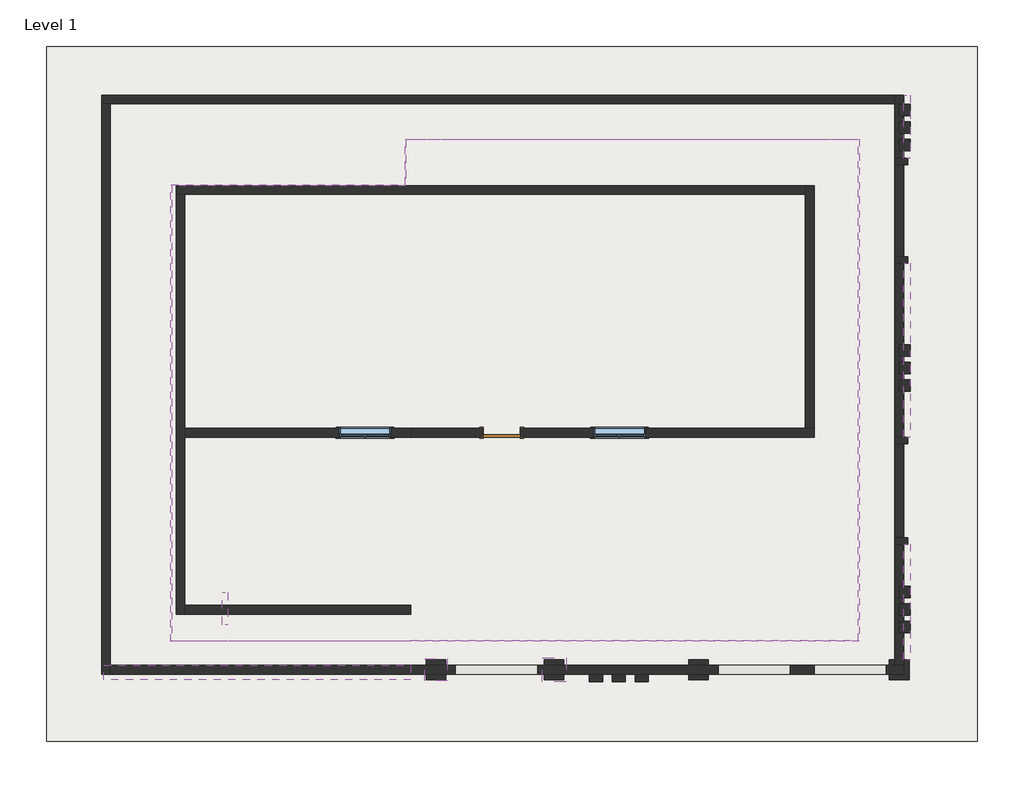
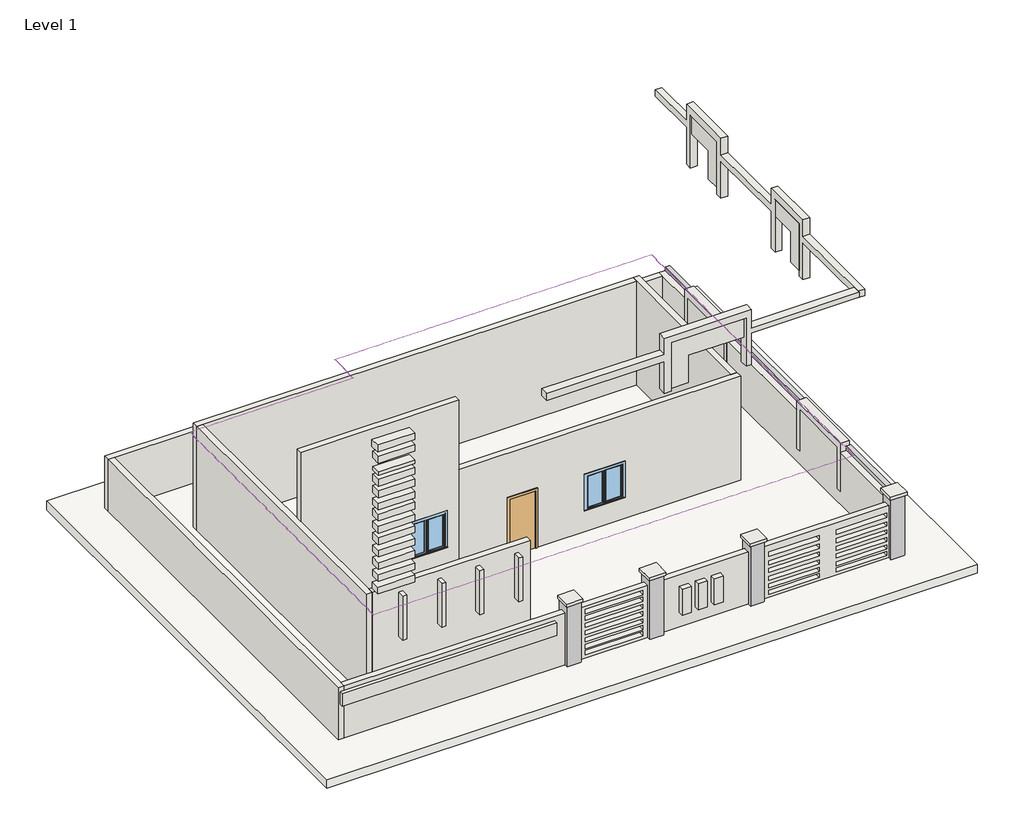
# One storey: 16 walls, 4 columns, 3 proxies, 2 coverings, 2 windows, 1 door, 1 slab.
"""IFC4 building model written with IfcOpenShell, lengths in millimetres."""

from ifc_helpers import new_model, si_unit, frame, origin, origin_with_axes, place, context, project, spatial, polyline, outline, extrude, faceted_brep, transform, mapped, element, save
from components import door_10fd3a06, walls_10_walls_10_12dc5ecd, walls_11_walls_11_b291a2b5, walls_12_walls_12_bacc6a5f, walls_13_walls_13_75e322be, walls_14_walls_14_a3be32cb, walls_2_walls_2_7a041f15, window_0862ab64

model = new_model("IFC4")

# Units and contexts
model_context = context("Model", 3, world=origin())
ifc_project = project(units=[si_unit("LENGTHUNIT", "METRE", prefix="MILLI")], contexts=[model_context])

# Site, building, storey
site = spatial("IfcSite", under=ifc_project)
building = spatial("IfcBuilding", under=site)
storey = spatial("IfcBuildingStorey", under=building, Name="Level 1", Elevation=0.0)

# Proxies
placement = place(None, origin())
element("IfcBuildingElementProxy", 1, Name="Cornice", ObjectType="Cornice", at=placement, inside=storey, context=model_context, shape_type="SweptSolid", body=[
    extrude(outline(polyline([(3201.2074298, -1465.8259649), (3353.6074298, -1465.8259649), (3353.6074298, -4158.7213241), (3201.2074298, -4158.7213241), (3201.2074298, -1465.8259649)])), frame((0.0, 0.0, 1828.8), z_axis=(0.0, 0.0, 1.0), x_axis=(1.0, 0.0, 0.0)), (0.0, 0.0, 1.0), 152.4),
])
element("IfcBuildingElementProxy", 2, Name="Cornice", ObjectType="Cornice", at=placement, inside=storey, context=model_context, shape_type="SweptSolid", body=[
    extrude(outline(polyline([(3201.2074298, 5061.9740351), (3353.6074298, 5061.9740351), (3353.6074298, 1023.3740351), (3201.2074298, 1023.3740351), (3201.2074298, 5061.9740351)])), frame((0.0, 0.0, 1828.8), z_axis=(0.0, 0.0, 1.0), x_axis=(1.0, 0.0, 0.0)), (0.0, 0.0, 1.0), 152.4),
])
element("IfcBuildingElementProxy", 3, Name="Cornice", ObjectType="Cornice", at=placement, inside=storey, context=model_context, shape_type="SweptSolid", body=[
    extrude(outline(polyline([(3201.2074298, 8973.0786759), (3353.6074298, 8973.0786759), (3353.6074298, 7499.8786759), (3201.2074298, 7499.8786759), (3201.2074298, 8973.0786759)])), frame((0.0, 0.0, 1785.441431), z_axis=(0.0, 0.0, 1.0), x_axis=(1.0, 0.0, 0.0)), (0.0, 0.0, 1.0), 152.4),
])

# Columns
element("IfcColumn", 4, ObjectType="Rectangular Column : 18\" x 18\"", at=placement, inside=storey, context=model_context, shape_type="SweptSolid", body=[
    extrude(outline(polyline([(-4615.9213241, 2133.6), (-4158.7213241, 2133.6), (-4158.7213241, 0.0), (-4285.7213241, 0.0), (-4285.7213241, 1828.8), (-4488.9213241, 1828.8), (-4488.9213241, 0.0), (-4615.9213241, 0.0), (-4615.9213241, 2133.6)])), frame((-7895.1305193, 0.0, 0.0), z_axis=(1.0, 0.0, 0.0), x_axis=(0.0, 1.0, 0.0)), (0.0, 0.0, 1.0), 457.2),
])
element("IfcColumn", 5, ObjectType="Rectangular Column : 18\" x 18\"", at=placement, inside=storey, context=model_context, shape_type="SweptSolid", body=[
    extrude(outline(polyline([(-4615.9213241, 2133.6), (-4158.7213241, 2133.6), (-4158.7213241, 0.0), (-4285.7213241, 0.0), (-4285.7213241, 1828.8), (-4488.9213241, 1828.8), (-4488.9213241, 0.0), (-4615.9213241, 0.0), (-4615.9213241, 2133.6)])), frame((-5151.9305193, 0.0, 0.0), z_axis=(1.0, 0.0, 0.0), x_axis=(0.0, 1.0, 0.0)), (0.0, 0.0, 1.0), 457.2),
])
element("IfcColumn", 6, ObjectType="Rectangular Column : 18\" x 18\"", at=placement, inside=storey, context=model_context, shape_type="SweptSolid", body=[
    extrude(outline(polyline([(-4615.9213241, 2133.6), (-4158.7213241, 2133.6), (-4158.7213241, 0.0), (-4285.7213241, 0.0), (-4285.7213241, 1828.8), (-4488.9213241, 1828.8), (-4488.9213241, 0.0), (-4615.9213241, 0.0), (-4615.9213241, 2133.6)])), frame((-1799.1305193, 0.0, 0.0), z_axis=(1.0, 0.0, 0.0), x_axis=(0.0, 1.0, 0.0)), (0.0, 0.0, 1.0), 457.2),
])
element("IfcColumn", 7, ObjectType="Rectangular Column : 18\" x 18\"", at=placement, inside=storey, context=model_context, shape_type="Brep", body=[
    faceted_brep([(3328.2074298, -4158.7213241, 2133.6), (2871.0074298, -4158.7213241, 2133.6), (2871.0074298, -4615.9213241, 2133.6), (3328.2074298, -4615.9213241, 2133.6), (2871.0074298, -4285.7213241, 0.0), (2871.0074298, -4158.7213241, 0.0), (2998.0074298, -4158.7213241, 0.0), (2998.0074298, -4285.7213241, 0.0), (3328.2074298, -4158.7213241, 0.0), (3201.2074298, -4158.7213241, 0.0), (3201.2074298, -4158.7213241, 1828.8), (2998.0074298, -4158.7213241, 1828.8), (2871.0074298, -4285.7213241, 1828.8), (2871.0074298, -4488.9213241, 1828.8), (2871.0074298, -4488.9213241, 0.0), (2871.0074298, -4615.9213241, 0.0), (3328.2074298, -4615.9213241, 0.0), (2998.0074298, -4285.7213241, 1828.8), (3201.2074298, -4488.9213241, 1828.8), (3201.2074298, -4488.9213241, 0.0), (3201.2074298, -4285.7213241, 1828.8), (3201.2074298, -4285.7213241, 0.0)], [[[0, 1, 2, 3]], [[4, 5, 6, 7]], [[1, 0, 8, 9, 10, 11, 6, 5]], [[2, 1, 5, 4, 12, 13, 14, 15]], [[3, 2, 15, 16]], [[0, 3, 16, 8]], [[12, 4, 7, 17]], [[18, 19, 14, 13]], [[19, 18, 20, 21]], [[11, 17, 7, 6]], [[20, 10, 9, 21]], [[8, 16, 15, 14, 19, 21, 9]], [[18, 13, 12, 17, 20]], [[17, 11, 10, 20]]]),
])

# Coverings
element("IfcCovering", 8, ObjectType="Fascia-Flat 1x12", at=placement, inside=storey, context=model_context, shape_type="Brep", body=[
    faceted_brep([(-8249.5228698, -3720.0759649, 3657.6), (-8249.5228698, -3707.3759649, 3657.6), (-8249.5228698, -3701.0259649, 3657.6), (-8249.5228698, -3701.0259649, 3371.85), (-8249.5228698, -3707.3759649, 3371.85), (-8249.5228698, -3720.0759649, 3371.85), (2164.4771302, -3720.0759649, 3657.6), (2145.4271302, -3701.0259649, 3657.6), (2145.4271302, -3701.0259649, 3371.85), (2164.4771302, -3720.0759649, 3371.85), (2164.4771302, 7951.2240351, 3657.6), (2145.4271302, 7932.1740351, 3657.6), (2145.4271302, 7932.1740351, 3371.85), (2164.4771302, 7951.2240351, 3371.85), (-8389.2228698, 7951.2240351, 3657.6), (-8370.1728698, 7932.1740351, 3657.6), (-8370.1728698, 7932.1740351, 3371.85), (-8389.2228698, 7951.2240351, 3371.85), (-8389.2228698, 6884.4240351, 3657.6), (-8370.1728698, 6865.3740351, 3657.6), (-8370.1728698, 6865.3740351, 3371.85), (-8389.2228698, 6884.4240351, 3371.85), (-13832.3805193, 6884.4240351, 3657.6), (-13813.3305193, 6865.3740351, 3657.6), (-13813.3305193, 6865.3740351, 3371.85), (-13832.3805193, 6884.4240351, 3371.85), (-13832.3805193, -3726.4259649, 3657.6), (-13832.3805193, -3726.4259649, 3371.85), (-13813.3305193, -3707.3759649, 3371.85), (-13813.3305193, -3707.3759649, 3657.6)], [[[0, 1, 2, 3, 4, 5]], [[2, 1, 0, 6, 7]], [[3, 2, 7, 8]], [[5, 4, 3, 8, 9]], [[0, 5, 9, 6]], [[7, 6, 10, 11]], [[8, 7, 11, 12]], [[9, 8, 12, 13]], [[6, 9, 13, 10]], [[11, 10, 14, 15]], [[12, 11, 15, 16]], [[13, 12, 16, 17]], [[10, 13, 17, 14]], [[15, 14, 18, 19]], [[16, 15, 19, 20]], [[17, 16, 20, 21]], [[14, 17, 21, 18]], [[19, 18, 22, 23]], [[20, 19, 23, 24]], [[21, 20, 24, 25]], [[18, 21, 25, 22]], [[26, 27, 28, 29]], [[23, 22, 26, 29]], [[24, 23, 29, 28]], [[25, 24, 28, 27]], [[22, 25, 27, 26]]]),
])
element("IfcCovering", 9, ObjectType="Fascia-Flat 1x12", at=placement, inside=storey, context=model_context, shape_type="Brep", body=[
    faceted_brep([(-13832.3805193, -3726.4259649, 3657.6), (-13813.3305193, -3707.3759649, 3657.6), (-13813.3305193, -3707.3759649, 3371.85), (-13832.3805193, -3726.4259649, 3371.85), (-8249.5228698, -3726.4259649, 3657.6), (-8249.5228698, -3726.4259649, 3371.85), (-8249.5228698, -3720.0759649, 3371.85), (-8249.5228698, -3707.3759649, 3371.85), (-8249.5228698, -3707.3759649, 3657.6), (-8249.5228698, -3720.0759649, 3657.6)], [[[0, 1, 2, 3]], [[4, 5, 6, 7, 8, 9]], [[1, 0, 4, 9, 8]], [[2, 1, 8, 7]], [[3, 2, 7, 6, 5]], [[0, 3, 5, 4]]]),
])

# Door
door_shape = door_10fd3a06(model_context)
element("IfcDoor", 10, ObjectType="Door-Single-Panel : 34\" x 80\"", at=placement, inside=storey, context=model_context, shape_type="MappedRepresentation", body=[
    mapped(door_shape, transform((-6142.5305193, 1124.9740351, 0.0), x_axis=(-1.0, 0.0, 0.0), y_axis=(0.0, -1.0, 0.0), z_axis=(0.0, 0.0, 1.0))),
])

# Slab
element("IfcSlab", 11, ObjectType="Generic - 12\"", at=placement, inside=storey, context=model_context, shape_type="SweptSolid", body=[
    extrude(outline(polyline([(4918.0010577, 10101.1985991), (4918.0010577, -6053.2014009), (-16722.7989423, -6053.2014009), (-16722.7989423, 10101.1985991), (4918.0010577, 10101.1985991)])), frame((0.0, 0.0, -304.8), z_axis=(0.0, 0.0, 1.0), x_axis=(1.0, 0.0, 0.0)), (0.0, 0.0, 1.0), 304.8),
])

# Walls
element("IfcWall", 12, ObjectType="Generic - 8\"", at=placement, inside=storey, context=model_context, shape_type="Brep", body=[
    faceted_brep([(-13711.7305193, 6662.1740351, 0.0), (-13508.5305193, 6662.1740351, 0.0), (918.6694807, 6662.1740351, 0.0), (918.6694807, 6662.1740351, 3657.6), (-13508.5305193, 6662.1740351, 3657.6), (-13711.7305193, 6662.1740351, 3657.6), (-13711.7305193, 6865.3740351, 0.0), (-13711.7305193, 6865.3740351, 3657.6), (-8370.1728698, 6865.3740351, 3657.6), (918.6694807, 6865.3740351, 3657.6), (918.6694807, 6865.3740351, 0.0)], [[[0, 1, 2, 3, 4, 5]], [[6, 7, 8, 9, 10]], [[2, 1, 0, 6, 10]], [[0, 5, 7, 6]], [[3, 2, 10, 9]], [[5, 4, 3, 9, 8, 7]]]),
])
element("IfcWall", 13, ObjectType="Generic - 8\"", at=placement, inside=storey, context=model_context, shape_type="Brep", body=[
    faceted_brep([(-13508.5305193, -3091.4259649, 0.0), (-13508.5305193, -2888.2259649, 0.0), (-13508.5305193, 1023.3740351, 0.0), (-13508.5305193, 1226.5740351, 0.0), (-13508.5305193, 6662.1740351, 0.0), (-13508.5305193, 6662.1740351, 3657.6), (-13508.5305193, -2888.2259649, 3657.6), (-13508.5305193, -3091.4259649, 3657.6), (-13711.7305193, -3091.4259649, 0.0), (-13711.7305193, -3091.4259649, 3657.6), (-13711.7305193, 6662.1740351, 3657.6), (-13711.7305193, 6662.1740351, 0.0)], [[[0, 1, 2, 3, 4, 5, 6, 7]], [[8, 9, 10, 11]], [[4, 3, 2, 1, 0, 8, 11]], [[0, 7, 9, 8]], [[5, 4, 11, 10]], [[7, 6, 5, 10, 9]]]),
])
element("IfcWall", 14, ObjectType="Generic - 8\"", at=placement, inside=storey, context=model_context, shape_type="SweptSolid", body=[
    extrude(outline(polyline([(-13508.5305193, -2888.2259649), (-8250.7305193, -2888.2259649), (-8250.7305193, -3091.4259649), (-13508.5305193, -3091.4259649), (-13508.5305193, -2888.2259649)])), origin_with_axes(), (0.0, 0.0, 1.0), 3657.6),
])
element("IfcWall", 15, ObjectType="Generic - 8\"", at=placement, inside=storey, context=model_context, shape_type="Brep", body=[
    faceted_brep([(918.6694807, 6865.3740351, 0.0), (918.6694807, 6662.1740351, 0.0), (918.6694807, 1226.5740351, 0.0), (918.6694807, 1226.5740351, 3657.6), (918.6694807, 6662.1740351, 3657.6), (918.6694807, 6865.3740351, 3657.6), (1121.8694807, 6865.3740351, 0.0), (1121.8694807, 6865.3740351, 3657.6), (1121.8694807, 1226.5740351, 3657.6), (1121.8694807, 1226.5740351, 0.0)], [[[0, 1, 2, 3, 4, 5]], [[6, 7, 8, 9]], [[2, 1, 0, 6, 9]], [[0, 5, 7, 6]], [[5, 4, 3, 8, 7]], [[3, 2, 9, 8]]]),
])
element("IfcWall", 16, ObjectType="Generic - 8\"", at=placement, inside=storey, context=model_context, shape_type="Brep", body=[
    faceted_brep([(-8250.7305193, 1023.3740351, 0.0), (-6574.3305193, 1023.3740351, 0.0), (-6574.3305193, 1023.3740351, 2032.0), (-5710.7305193, 1023.3740351, 2032.0), (-5710.7305193, 1023.3740351, 0.0), (1121.8694807, 1023.3740351, 0.0), (1121.8694807, 1023.3740351, 3657.6), (-8250.7305193, 1023.3740351, 3657.6), (-4008.9305193, 1023.3740351, 1960.9254934), (-2789.7305193, 1023.3740351, 1960.9254934), (-2789.7305193, 1023.3740351, 741.7254934), (-4008.9305193, 1023.3740351, 741.7254934), (-6574.3305193, 1226.5740351, 2032.0), (-6574.3305193, 1226.5740351, 0.0), (-8250.7305193, 1226.5740351, 0.0), (-8250.7305193, 1226.5740351, 3657.6), (918.6694807, 1226.5740351, 3657.6), (1121.8694807, 1226.5740351, 3657.6), (1121.8694807, 1226.5740351, 0.0), (918.6694807, 1226.5740351, 0.0), (-5710.7305193, 1226.5740351, 0.0), (-5710.7305193, 1226.5740351, 2032.0), (-4008.9305193, 1226.5740351, 1960.9254934), (-4008.9305193, 1226.5740351, 741.7254934), (-2789.7305193, 1226.5740351, 741.7254934), (-2789.7305193, 1226.5740351, 1960.9254934)], [[[0, 1, 2, 3, 4, 5, 6, 7], [8, 9, 10, 11]], [[12, 13, 14, 15, 16, 17, 18, 19, 20, 21], [22, 23, 24, 25]], [[14, 13, 1, 0]], [[20, 19, 18, 5, 4]], [[7, 6, 17, 16, 15]], [[0, 7, 15, 14]], [[6, 5, 18, 17]], [[23, 22, 8, 11]], [[24, 23, 11, 10]], [[25, 24, 10, 9]], [[22, 25, 9, 8]], [[2, 1, 13, 12]], [[3, 2, 12, 21]], [[4, 3, 21, 20]]]),
])
element("IfcWall", 17, ObjectType="Generic - 8\"", at=placement, inside=storey, context=model_context, shape_type="Brep", body=[
    faceted_brep([(-8250.7305193, 1226.5740351, 0.0), (-13508.5305193, 1226.5740351, 0.0), (-13508.5305193, 1226.5740351, 6096.0), (-8250.7305193, 1226.5740351, 6096.0), (-8250.7305193, 1226.5740351, 3657.6), (-9927.1305193, 1226.5740351, 2285.1492606), (-9927.1305193, 1226.5740351, 1065.9492606), (-8707.9305193, 1226.5740351, 1065.9492606), (-8707.9305193, 1226.5740351, 2285.1492606), (-8250.7305193, 1023.3740351, 0.0), (-8250.7305193, 1023.3740351, 3657.6), (-8250.7305193, 1023.3740351, 6096.0), (-13508.5305193, 1023.3740351, 6096.0), (-13508.5305193, 1023.3740351, 0.0), (-9927.1305193, 1023.3740351, 2285.1492606), (-8707.9305193, 1023.3740351, 2285.1492606), (-8707.9305193, 1023.3740351, 1065.9492606), (-9927.1305193, 1023.3740351, 1065.9492606)], [[[0, 1, 2, 3, 4], [5, 6, 7, 8]], [[9, 10, 11, 12, 13], [14, 15, 16, 17]], [[1, 0, 9, 13]], [[3, 2, 12, 11]], [[0, 4, 3, 11, 10, 9]], [[2, 1, 13, 12]], [[6, 5, 14, 17]], [[7, 6, 17, 16]], [[8, 7, 16, 15]], [[5, 8, 15, 14]]]),
])
element("IfcWall", 18, ObjectType="Generic - 8\"", at=placement, inside=storey, context=model_context, shape_type="Brep", body=[
    faceted_brep([(-15442.3925702, 8769.8786759, 0.0), (-15239.1925702, 8769.8786759, 0.0), (2998.0074298, 8769.8786759, 0.0), (2998.0074298, 8769.8786759, 1828.8), (-15239.1925702, 8769.8786759, 1828.8), (-15442.3925702, 8769.8786759, 1828.8), (-15442.3925702, 8973.0786759, 0.0), (-15442.3925702, 8973.0786759, 1828.8), (2998.0074298, 8973.0786759, 1828.8), (2998.0074298, 8973.0786759, 0.0)], [[[0, 1, 2, 3, 4, 5]], [[6, 7, 8, 9]], [[2, 1, 0, 6, 9]], [[5, 4, 3, 8, 7]], [[0, 5, 7, 6]], [[3, 2, 9, 8]]]),
])
element("IfcWall", 19, ObjectType="Generic - 8\"", at=placement, inside=storey, context=model_context, shape_type="Brep", body=[
    faceted_brep([(-15239.1925702, -4488.9213241, 0.0), (-15239.1925702, -4285.7213241, 0.0), (-15239.1925702, 8769.8786759, 0.0), (-15239.1925702, 8769.8786759, 1828.8), (-15239.1925702, -4285.7213241, 1828.8), (-15239.1925702, -4488.9213241, 1828.8), (-15442.3925702, -4488.9213241, 0.0), (-15442.3925702, -4488.9213241, 1828.8), (-15442.3925702, 8769.8786759, 1828.8), (-15442.3925702, 8769.8786759, 0.0)], [[[0, 1, 2, 3, 4, 5]], [[6, 7, 8, 9]], [[2, 1, 0, 6, 9]], [[5, 4, 3, 8, 7]], [[0, 5, 7, 6]], [[3, 2, 9, 8]]]),
])
element("IfcWall", 20, ObjectType="Generic - 8\"", at=placement, inside=storey, context=model_context, shape_type="Brep", body=[
    faceted_brep([(3201.2074298, -4285.7213241, 0.0), (2998.0074298, -4285.7213241, 0.0), (2871.0074298, -4285.7213241, 0.0), (-1341.9305193, -4285.7213241, 0.0), (-1799.1305193, -4285.7213241, 0.0), (-4694.7305193, -4285.7213241, 0.0), (-5151.9305193, -4285.7213241, 0.0), (-7437.9305193, -4285.7213241, 0.0), (-7895.1305193, -4285.7213241, 0.0), (-15239.1925702, -4285.7213241, 0.0), (-15239.1925702, -4285.7213241, 1828.8), (-7895.1305193, -4285.7213241, 1828.8), (-7437.9305193, -4285.7213241, 1828.8), (-5151.9305193, -4285.7213241, 1828.8), (-4694.7305193, -4285.7213241, 1828.8), (-1799.1305193, -4285.7213241, 1828.8), (-1341.9305193, -4285.7213241, 1828.8), (2871.0074298, -4285.7213241, 1828.8), (2998.0074298, -4285.7213241, 1828.8), (3201.2074298, -4285.7213241, 1828.8), (2798.2694807, -4285.7213241, 1590.6295089), (1121.8694807, -4285.7213241, 1590.6295089), (1121.8694807, -4285.7213241, 1438.2295089), (2798.2694807, -4285.7213241, 1438.2295089), (2798.2694807, -4285.7213241, 1285.530341), (1121.8694807, -4285.7213241, 1285.530341), (1121.8694807, -4285.7213241, 1133.7858691), (2798.2694807, -4285.7213241, 1133.7858691), (2798.2694807, -4285.7213241, 1009.753772), (1121.8694807, -4285.7213241, 1009.753772), (1121.8694807, -4285.7213241, 869.7393415), (2798.2694807, -4285.7213241, 869.7393415), (2798.2694807, -4285.7213241, 736.2637339), (1121.8694807, -4285.7213241, 736.2637339), (1121.8694807, -4285.7213241, 596.2533887), (2798.2694807, -4285.7213241, 596.2533887), (2798.2694807, -4285.7213241, 467.4688962), (1121.8694807, -4285.7213241, 467.4688962), (1121.8694807, -4285.7213241, 327.4258682), (2798.2694807, -4285.7213241, 327.4258682), (2798.2694807, -4285.7213241, 250.5459581), (1121.8694807, -4285.7213241, 250.5459581), (1121.8694807, -4285.7213241, 105.8322418), (2798.2694807, -4285.7213241, 105.8322418), (563.0694807, -4285.7213241, 1590.6295089), (-1113.3305193, -4285.7213241, 1590.6295089), (-1113.3305193, -4285.7213241, 1438.2295089), (563.0694807, -4285.7213241, 1438.2295089), (563.0694807, -4285.7213241, 1285.530341), (-1113.3305193, -4285.7213241, 1285.530341), (-1113.3305193, -4285.7213241, 1133.7858691), (563.0694807, -4285.7213241, 1133.7858691), (563.0694807, -4285.7213241, 1009.753772), (-1113.3305193, -4285.7213241, 1009.753772), (-1113.3305193, -4285.7213241, 869.7393415), (563.0694807, -4285.7213241, 869.7393415), (563.0694807, -4285.7213241, 736.2637339), (-1113.3305193, -4285.7213241, 736.2637339), (-1113.3305193, -4285.7213241, 596.2533887), (563.0694807, -4285.7213241, 596.2533887), (563.0694807, -4285.7213241, 467.4688962), (-1113.3305193, -4285.7213241, 467.4688962), (-1113.3305193, -4285.7213241, 327.4258682), (563.0694807, -4285.7213241, 327.4258682), (563.0694807, -4285.7213241, 250.5459581), (-1113.3305193, -4285.7213241, 250.5459581), (-1113.3305193, -4285.7213241, 105.8322418), (563.0694807, -4285.7213241, 105.8322418), (-5305.1552948, -4285.7213241, 1704.9295089), (-7219.390028, -4285.7213241, 1704.9295089), (-7219.390028, -4285.7213241, 1552.5295089), (-5305.1552948, -4285.7213241, 1552.5295089), (-5305.1552948, -4285.7213241, 1225.653772), (-7219.390028, -4285.7213241, 1225.653772), (-7219.390028, -4285.7213241, 1073.253772), (-5305.1552948, -4285.7213241, 1073.253772), (-5305.1552948, -4285.7213241, 964.8637339), (-7219.390028, -4285.7213241, 964.8637339), (-7219.390028, -4285.7213241, 812.4637339), (-5305.1552948, -4285.7213241, 812.4637339), (-5305.1552948, -4285.7213241, 715.1188962), (-7219.390028, -4285.7213241, 715.1188962), (-7219.390028, -4285.7213241, 562.7188962), (-5305.1552948, -4285.7213241, 562.7188962), (-5305.1552948, -4285.7213241, 479.1459581), (-7219.390028, -4285.7213241, 479.1459581), (-7219.390028, -4285.7213241, 326.7459581), (-5305.1552948, -4285.7213241, 326.7459581), (-5305.1552948, -4285.7213241, 1476.3295089), (-7219.390028, -4285.7213241, 1476.3295089), (-7219.390028, -4285.7213241, 1323.9295089), (-5305.1552948, -4285.7213241, 1323.9295089), (-5305.1552948, -4285.7213241, 263.2459581), (-7219.390028, -4285.7213241, 263.2459581), (-7219.390028, -4285.7213241, 110.8459581), (-5305.1552948, -4285.7213241, 110.8459581), (3201.2074298, -4488.9213241, 0.0), (3201.2074298, -4488.9213241, 1828.8), (2871.0074298, -4488.9213241, 1828.8), (-1341.9305193, -4488.9213241, 1828.8), (-1799.1305193, -4488.9213241, 1828.8), (-4694.7305193, -4488.9213241, 1828.8), (-5151.9305193, -4488.9213241, 1828.8), (-7437.9305193, -4488.9213241, 1828.8), (-7895.1305193, -4488.9213241, 1828.8), (-15239.1925702, -4488.9213241, 1828.8), (-15239.1925702, -4488.9213241, 0.0), (-7895.1305193, -4488.9213241, 0.0), (-7437.9305193, -4488.9213241, 0.0), (-5151.9305193, -4488.9213241, 0.0), (-4694.7305193, -4488.9213241, 0.0), (-1799.1305193, -4488.9213241, 0.0), (-1341.9305193, -4488.9213241, 0.0), (2871.0074298, -4488.9213241, 0.0), (2798.2694807, -4488.9213241, 1590.6295089), (2798.2694807, -4488.9213241, 1438.2295089), (1121.8694807, -4488.9213241, 1438.2295089), (1121.8694807, -4488.9213241, 1590.6295089), (2798.2694807, -4488.9213241, 1285.530341), (2798.2694807, -4488.9213241, 1133.7858691), (1121.8694807, -4488.9213241, 1133.7858691), (1121.8694807, -4488.9213241, 1285.530341), (2798.2694807, -4488.9213241, 1009.753772), (2798.2694807, -4488.9213241, 869.7393415), (1121.8694807, -4488.9213241, 869.7393415), (1121.8694807, -4488.9213241, 1009.753772), (2798.2694807, -4488.9213241, 736.2637339), (2798.2694807, -4488.9213241, 596.2533887), (1121.8694807, -4488.9213241, 596.2533887), (1121.8694807, -4488.9213241, 736.2637339), (2798.2694807, -4488.9213241, 467.4688962), (2798.2694807, -4488.9213241, 327.4258682), (1121.8694807, -4488.9213241, 327.4258682), (1121.8694807, -4488.9213241, 467.4688962), (2798.2694807, -4488.9213241, 250.5459581), (2798.2694807, -4488.9213241, 105.8322418), (1121.8694807, -4488.9213241, 105.8322418), (1121.8694807, -4488.9213241, 250.5459581), (563.0694807, -4488.9213241, 1590.6295089), (563.0694807, -4488.9213241, 1438.2295089), (-1113.3305193, -4488.9213241, 1438.2295089), (-1113.3305193, -4488.9213241, 1590.6295089), (563.0694807, -4488.9213241, 1285.530341), (563.0694807, -4488.9213241, 1133.7858691), (-1113.3305193, -4488.9213241, 1133.7858691), (-1113.3305193, -4488.9213241, 1285.530341), (563.0694807, -4488.9213241, 1009.753772), (563.0694807, -4488.9213241, 869.7393415), (-1113.3305193, -4488.9213241, 869.7393415), (-1113.3305193, -4488.9213241, 1009.753772), (563.0694807, -4488.9213241, 736.2637339), (563.0694807, -4488.9213241, 596.2533887), (-1113.3305193, -4488.9213241, 596.2533887), (-1113.3305193, -4488.9213241, 736.2637339), (563.0694807, -4488.9213241, 467.4688962), (563.0694807, -4488.9213241, 327.4258682), (-1113.3305193, -4488.9213241, 327.4258682), (-1113.3305193, -4488.9213241, 467.4688962), (563.0694807, -4488.9213241, 250.5459581), (563.0694807, -4488.9213241, 105.8322418), (-1113.3305193, -4488.9213241, 105.8322418), (-1113.3305193, -4488.9213241, 250.5459581), (-5305.1552948, -4488.9213241, 1704.9295089), (-5305.1552948, -4488.9213241, 1552.5295089), (-7219.390028, -4488.9213241, 1552.5295089), (-7219.390028, -4488.9213241, 1704.9295089), (-5305.1552948, -4488.9213241, 1225.653772), (-5305.1552948, -4488.9213241, 1073.253772), (-7219.390028, -4488.9213241, 1073.253772), (-7219.390028, -4488.9213241, 1225.653772), (-5305.1552948, -4488.9213241, 964.8637339), (-5305.1552948, -4488.9213241, 812.4637339), (-7219.390028, -4488.9213241, 812.4637339), (-7219.390028, -4488.9213241, 964.8637339), (-5305.1552948, -4488.9213241, 715.1188962), (-5305.1552948, -4488.9213241, 562.7188962), (-7219.390028, -4488.9213241, 562.7188962), (-7219.390028, -4488.9213241, 715.1188962), (-5305.1552948, -4488.9213241, 479.1459581), (-5305.1552948, -4488.9213241, 326.7459581), (-7219.390028, -4488.9213241, 326.7459581), (-7219.390028, -4488.9213241, 479.1459581), (-5305.1552948, -4488.9213241, 1476.3295089), (-5305.1552948, -4488.9213241, 1323.9295089), (-7219.390028, -4488.9213241, 1323.9295089), (-7219.390028, -4488.9213241, 1476.3295089), (-5305.1552948, -4488.9213241, 263.2459581), (-5305.1552948, -4488.9213241, 110.8459581), (-7219.390028, -4488.9213241, 110.8459581), (-7219.390028, -4488.9213241, 263.2459581)], [[[0, 1, 2, 3, 4, 5, 6, 7, 8, 9, 10, 11, 12, 13, 14, 15, 16, 17, 18, 19], [20, 21, 22, 23], [24, 25, 26, 27], [28, 29, 30, 31], [32, 33, 34, 35], [36, 37, 38, 39], [40, 41, 42, 43], [44, 45, 46, 47], [48, 49, 50, 51], [52, 53, 54, 55], [56, 57, 58, 59], [60, 61, 62, 63], [64, 65, 66, 67], [68, 69, 70, 71], [72, 73, 74, 75], [76, 77, 78, 79], [80, 81, 82, 83], [84, 85, 86, 87], [88, 89, 90, 91], [92, 93, 94, 95]], [[96, 97, 98, 99, 100, 101, 102, 103, 104, 105, 106, 107, 108, 109, 110, 111, 112, 113], [114, 115, 116, 117], [118, 119, 120, 121], [122, 123, 124, 125], [126, 127, 128, 129], [130, 131, 132, 133], [134, 135, 136, 137], [138, 139, 140, 141], [142, 143, 144, 145], [146, 147, 148, 149], [150, 151, 152, 153], [154, 155, 156, 157], [158, 159, 160, 161], [162, 163, 164, 165], [166, 167, 168, 169], [170, 171, 172, 173], [174, 175, 176, 177], [178, 179, 180, 181], [182, 183, 184, 185], [186, 187, 188, 189]], [[0, 19, 97, 96]], [[10, 9, 106, 105]], [[9, 8, 7, 6, 5, 4, 3, 2, 1, 0, 96, 113, 112, 111, 110, 109, 108, 107, 106]], [[19, 18, 17, 16, 15, 14, 13, 12, 11, 10, 105, 104, 103, 102, 101, 100, 99, 98, 97]], [[21, 20, 114, 117]], [[22, 21, 117, 116]], [[23, 22, 116, 115]], [[20, 23, 115, 114]], [[25, 24, 118, 121]], [[26, 25, 121, 120]], [[27, 26, 120, 119]], [[24, 27, 119, 118]], [[29, 28, 122, 125]], [[30, 29, 125, 124]], [[31, 30, 124, 123]], [[28, 31, 123, 122]], [[33, 32, 126, 129]], [[34, 33, 129, 128]], [[35, 34, 128, 127]], [[32, 35, 127, 126]], [[37, 36, 130, 133]], [[38, 37, 133, 132]], [[39, 38, 132, 131]], [[36, 39, 131, 130]], [[41, 40, 134, 137]], [[42, 41, 137, 136]], [[43, 42, 136, 135]], [[40, 43, 135, 134]], [[45, 44, 138, 141]], [[46, 45, 141, 140]], [[47, 46, 140, 139]], [[44, 47, 139, 138]], [[49, 48, 142, 145]], [[50, 49, 145, 144]], [[51, 50, 144, 143]], [[48, 51, 143, 142]], [[53, 52, 146, 149]], [[54, 53, 149, 148]], [[55, 54, 148, 147]], [[52, 55, 147, 146]], [[57, 56, 150, 153]], [[58, 57, 153, 152]], [[59, 58, 152, 151]], [[56, 59, 151, 150]], [[61, 60, 154, 157]], [[62, 61, 157, 156]], [[63, 62, 156, 155]], [[60, 63, 155, 154]], [[65, 64, 158, 161]], [[66, 65, 161, 160]], [[67, 66, 160, 159]], [[64, 67, 159, 158]], [[69, 68, 162, 165]], [[70, 69, 165, 164]], [[71, 70, 164, 163]], [[68, 71, 163, 162]], [[73, 72, 166, 169]], [[74, 73, 169, 168]], [[75, 74, 168, 167]], [[72, 75, 167, 166]], [[77, 76, 170, 173]], [[78, 77, 173, 172]], [[79, 78, 172, 171]], [[76, 79, 171, 170]], [[81, 80, 174, 177]], [[82, 81, 177, 176]], [[83, 82, 176, 175]], [[80, 83, 175, 174]], [[85, 84, 178, 181]], [[86, 85, 181, 180]], [[87, 86, 180, 179]], [[84, 87, 179, 178]], [[89, 88, 182, 185]], [[90, 89, 185, 184]], [[91, 90, 184, 183]], [[88, 91, 183, 182]], [[93, 92, 186, 189]], [[94, 93, 189, 188]], [[95, 94, 188, 187]], [[92, 95, 187, 186]]]),
])
element("IfcWall", 21, ObjectType="Generic - 8\"", at=placement, inside=storey, context=model_context, shape_type="Brep", body=[
    faceted_brep([(2998.0074298, 8973.0786759, 0.0), (2998.0074298, 8769.8786759, 0.0), (2998.0074298, -4158.7213241, 0.0), (2998.0074298, -4285.7213241, 0.0), (2998.0074298, -4285.7213241, 1828.8), (2998.0074298, -4158.7213241, 1828.8), (2998.0074298, -1465.8259649, 1828.8), (2998.0074298, -1465.8259649, 2133.6), (2998.0074298, 1023.3740351, 2133.6), (2998.0074298, 1023.3740351, 1828.8), (2998.0074298, 5061.4786759, 1828.8), (2998.0074298, 5061.4786759, 2133.6), (2998.0074298, 7499.8786759, 2133.6), (2998.0074298, 7499.8786759, 1828.8), (2998.0074298, 8769.8786759, 1828.8), (2998.0074298, 8973.0786759, 1828.8), (3201.2074298, 8973.0786759, 0.0), (3201.2074298, 8973.0786759, 1828.8), (3201.2074298, 7499.8786759, 1828.8), (3201.2074298, 7499.8786759, 2133.6), (3201.2074298, 5061.4786759, 2133.6), (3201.2074298, 5061.4786759, 1828.8), (3201.2074298, 1023.3740351, 1828.8), (3201.2074298, 1023.3740351, 2133.6), (3201.2074298, -1465.8259649, 2133.6), (3201.2074298, -1465.8259649, 1828.8), (3201.2074298, -4158.7213241, 1828.8), (3201.2074298, -4285.7213241, 1828.8), (3201.2074298, -4285.7213241, 0.0), (3201.2074298, -4158.7213241, 0.0)], [[[0, 1, 2, 3, 4, 5, 6, 7, 8, 9, 10, 11, 12, 13, 14, 15]], [[16, 17, 18, 19, 20, 21, 22, 23, 24, 25, 26, 27, 28, 29]], [[0, 15, 17, 16]], [[4, 3, 28, 27]], [[3, 2, 1, 0, 16, 29, 28]], [[6, 5, 4, 27, 26, 25]], [[7, 6, 25, 24]], [[8, 7, 24, 23]], [[9, 8, 23, 22]], [[10, 9, 22, 21]], [[11, 10, 21, 20]], [[12, 11, 20, 19]], [[13, 12, 19, 18]], [[15, 14, 13, 18, 17]]]),
])
walls_10_walls_10_shape = walls_10_walls_10_12dc5ecd(model_context)
element("IfcWall", 22, ObjectType="Walls 10 : Walls 10", at=placement, inside=storey, context=model_context, shape_type="MappedRepresentation", body=[
    mapped(walls_10_walls_10_shape, transform((0.0, 0.0, 0.0), x_axis=(1.0, 0.0, 0.0), y_axis=(0.0, 1.0, 0.0), z_axis=(0.0, 0.0, 1.0))),
])
walls_11_walls_11_shape = walls_11_walls_11_b291a2b5(model_context)
element("IfcWall", 23, ObjectType="Walls 11 : Walls 11", at=placement, inside=storey, context=model_context, shape_type="MappedRepresentation", body=[
    mapped(walls_11_walls_11_shape, transform((0.0, 0.0, 0.0), x_axis=(1.0, 0.0, 0.0), y_axis=(0.0, 1.0, 0.0), z_axis=(0.0, 0.0, 1.0))),
])
walls_12_walls_12_shape = walls_12_walls_12_bacc6a5f(model_context)
element("IfcWall", 24, ObjectType="Walls 12 : Walls 12", at=placement, inside=storey, context=model_context, shape_type="MappedRepresentation", body=[
    mapped(walls_12_walls_12_shape, transform((0.0, 0.0, 0.0), x_axis=(1.0, 0.0, 0.0), y_axis=(0.0, 1.0, 0.0), z_axis=(0.0, 0.0, 1.0))),
])
walls_13_walls_13_shape = walls_13_walls_13_75e322be(model_context)
element("IfcWall", 25, ObjectType="Walls 13 : Walls 13", at=placement, inside=storey, context=model_context, shape_type="MappedRepresentation", body=[
    mapped(walls_13_walls_13_shape, transform((0.0, 0.0, 0.0), x_axis=(1.0, 0.0, 0.0), y_axis=(0.0, 1.0, 0.0), z_axis=(0.0, 0.0, 1.0))),
])
walls_14_walls_14_shape = walls_14_walls_14_a3be32cb(model_context)
element("IfcWall", 26, ObjectType="Walls 14 : Walls 14", at=placement, inside=storey, context=model_context, shape_type="MappedRepresentation", body=[
    mapped(walls_14_walls_14_shape, transform((0.0, 0.0, 0.0), x_axis=(1.0, 0.0, 0.0), y_axis=(0.0, 1.0, 0.0), z_axis=(0.0, 0.0, 1.0))),
])
walls_2_walls_2_shape = walls_2_walls_2_7a041f15(model_context)
element("IfcWall", 27, ObjectType="Walls 2 : Walls 2", at=placement, inside=storey, context=model_context, shape_type="MappedRepresentation", body=[
    mapped(walls_2_walls_2_shape, transform((0.0, 0.0, 0.0), x_axis=(1.0, 0.0, 0.0), y_axis=(0.0, 1.0, 0.0), z_axis=(0.0, 0.0, 1.0))),
])

# Windows
window_shape = window_0862ab64(model_context)
element("IfcWindow", 28, ObjectType="Casement Dbl with Trim : 48\" x 48\"", at=placement, inside=storey, context=model_context, shape_type="MappedRepresentation", body=[
    mapped(window_shape, transform((-3399.3305193, 1144.0240351, -172.6745066), x_axis=(-1.0, 0.0, 0.0), y_axis=(0.0, -1.0, 0.0), z_axis=(0.0, 0.0, 1.0))),
])
element("IfcWindow", 29, ObjectType="Casement Dbl with Trim : 48\" x 48\"", at=placement, inside=storey, context=model_context, shape_type="MappedRepresentation", body=[
    mapped(window_shape, transform((-9317.5305193, 1144.0240351, 151.5492606), x_axis=(-1.0, 0.0, 0.0), y_axis=(0.0, -1.0, 0.0), z_axis=(0.0, 0.0, 1.0))),
])

save(model, "model.ifc")

# Revit data of these elements
# Type "Rectangular Column : 18\" x 18\""
#   Assembly Code = "B1010200"
#   Depth = 1' - 6"
#   Offset Base = 0' - 0"
#   Offset Top = 0' - 0"
#   Width = 1' - 6"
#   Material = none
# Type "Door-Single-Panel : 34\" x 80\""
#   Type Mark = "8"
#   Construction Type Id = "DOOR"
#   Assembly Code = "C1020300"
#   Analytic Construction = "Wooden"
#   Thickness = 0' - 2"
#   Thermal Resistance (R) = 2.5876 (h·ft²·°F)/BTU
#   Swing Angle [instance default] = 90.00°
#   Heat Transfer Coefficient (U) = 0.3865 BTU/(h·ft²·°F)
#   Height = 6' - 8"
#   Trim Projection Ext = 0' - 1"
#   Trim Projection Int = 0' - 1"
#   Trim Width = 0' - 3"
#   Width = 2' - 10"
#   Define Thermal Properties by = 1
#   Panel Material = Wood - Birch - Solid Stained Light Low Gloss
#   Trim Material = Roofing, EPDM Membrane
#   Visual Light Transmittance = 0
#   Solar Heat Gain Coefficient = 0
#   Function = (empty or 0)
#   Wall Closure = (empty or 0)
# Type "Generic - 12\""
#   Assembly Code = "B1010"
#   Function = 0
#   Layers, outside or top first: 1' - 0" no material (function 1)
# Type "Generic - 8\""
#   Assembly Code = "B2010"
#   Layers, outside or top first: 0' - 8" no material (function 1)
# Type "Casement Dbl with Trim : 48\" x 48\""
#   Type Mark = "19"
#   Construction Type Id = "GSP4R"
#   Assembly Code = "B2020100"
#   Analytic Construction = "1/8 in Pilkington single glazing"
#   Visual Light Transmittance = 0.9
#   Solar Heat Gain Coefficient = 0.78
#   Heat Transfer Coefficient (U) = 0.6496 BTU/(h·ft²·°F)
#   Height = 4' - 0"
#   Default Sill Height = 3' - 0"
#   Trim Projection - Ext. = 0' - 0 1/2"
#   Trim Projection - Int. = 0' - 0 3/4"
#   Trim Width - Exterior = 0' - 3 1/2"
#   Trim Width - Interior = 0' - 3 1/2"
#   Width = 4' - 0"
#   Window Inset = 0' - 0 3/4"
#   Define Thermal Properties by = 1
#   Glass Pane Material = Glass
#   Sash Material = Sash
#   Trim Exterior Material = Trim
#   Trim Interior Material = Trim
#   Wall Closure = (empty or 0)
# Elements 1, 2, 3 (IfcBuildingElementProxy, "Cornice")
#   Phase Created = New Construction
#   Materials on its faces: "Default Wall"
# Elements 4, 5, 6, 7 (IfcColumn, "Rectangular Column : 18\" x 18\"")
#   Phase Created = New Construction
#   Materials on its faces: "Default Wall"
# Elements 8, 9 (IfcCovering, "Fascia-Flat 1x12")
#   Phase Created = New Construction
#   Materials on its faces: "Default Roof"
# Element 10 (IfcDoor, "Door-Single-Panel : 34\" x 80\"")
#   Swing Angle = 90.00°
#   Phase Created = New Construction
#   Materials on its faces: "Roofing, EPDM Membrane", "Wood - Birch - Solid Stained Light Low Gloss"
# Element 11 (IfcSlab, "Generic - 12\"")
#   Height Offset From Level = 0' - 0"
#   Phase Created = New Construction
#   Materials on its faces: "Default Floor"
# Elements 12, 13, 14, 15, 16 (IfcWall, "Generic - 8\"")
#   Top Offset = 0' - 0"
#   Base Offset = 0' - 0"
#   Unconnected Height = 12' - 0"
#   wall height = 12' - 0"
#   Phase Created = New Construction
#   Base Constraint = Level 1
#   Materials on its faces: "Default Wall"
# Element 17 (IfcWall, "Generic - 8\"")
#   Top Offset = 0' - 0"
#   Base Offset = 0' - 0"
#   Unconnected Height = 20' - 0"
#   wall height = 20' - 0"
#   Phase Created = New Construction
#   Base Constraint = Level 1
#   Materials on its faces: "Default Wall"
# Elements 18, 19, 20, 21 (IfcWall, "Generic - 8\"")
#   Top Offset = 0' - 0"
#   Base Offset = 0' - 0"
#   Unconnected Height = 6' - 0"
#   wall height = 6' - 0"
#   Phase Created = New Construction
#   Base Constraint = Level 1
#   Materials on its faces: "Default Wall"
# Element 22 (IfcWall, "Walls 10 : Walls 10")
#   Phase Created = New Construction
#   Materials on its faces: "Default Wall"
# Element 23 (IfcWall, "Walls 11 : Walls 11")
#   Phase Created = New Construction
#   Materials on its faces: "Default Wall"
# Element 24 (IfcWall, "Walls 12 : Walls 12")
#   Phase Created = New Construction
#   Materials on its faces: "Default Wall"
# Element 25 (IfcWall, "Walls 13 : Walls 13")
#   Phase Created = New Construction
#   Materials on its faces: "Default Wall"
# Element 26 (IfcWall, "Walls 14 : Walls 14")
#   Phase Created = New Construction
#   Materials on its faces: "Brick, Common"
# Element 27 (IfcWall, "Walls 2 : Walls 2")
#   Phase Created = New Construction
#   Materials on its faces: "Default Wall"
# Element 28 (IfcWindow, "Casement Dbl with Trim : 48\" x 48\"")
#   Mark = "5"
#   Phase Created = New Construction
#   Materials on its faces: "Sash", "Trim", "Glass"
# Element 29 (IfcWindow, "Casement Dbl with Trim : 48\" x 48\"")
#   Mark = "6"
#   Phase Created = New Construction
#   Materials on its faces: "Sash", "Trim", "Glass"
# Materials
#   "Wood - Birch - Solid Stained Light Low Gloss": class "Wood", colour RGB 210 159 95, transparency 0, Cost = 0
#   "Roofing, EPDM Membrane": class "Generic", colour RGB 127 127 127, transparency 0, Description = "EPDM roof membrane", Cost = 0
#   "Glass": class "Glass", colour RGB 0 128 192, transparency 0.75, Description = "Soda Lime Glass", Cost = 0
#   "Sash": class "Wood", colour RGB 224 178 126, transparency 0
#   "Trim": class "Wood", colour RGB 224 178 126, transparency 0
#   "Default Wall": colour RGB 128 128 128, transparency 0
#   "Default Roof": colour RGB 88 101 114, transparency 0
#   "Default Floor": colour RGB 128 128 128, transparency 0
#   "Brick, Common": class "Masonry", colour RGB 0 0 0, transparency 0, Description = "Common brick", Cost = 0
